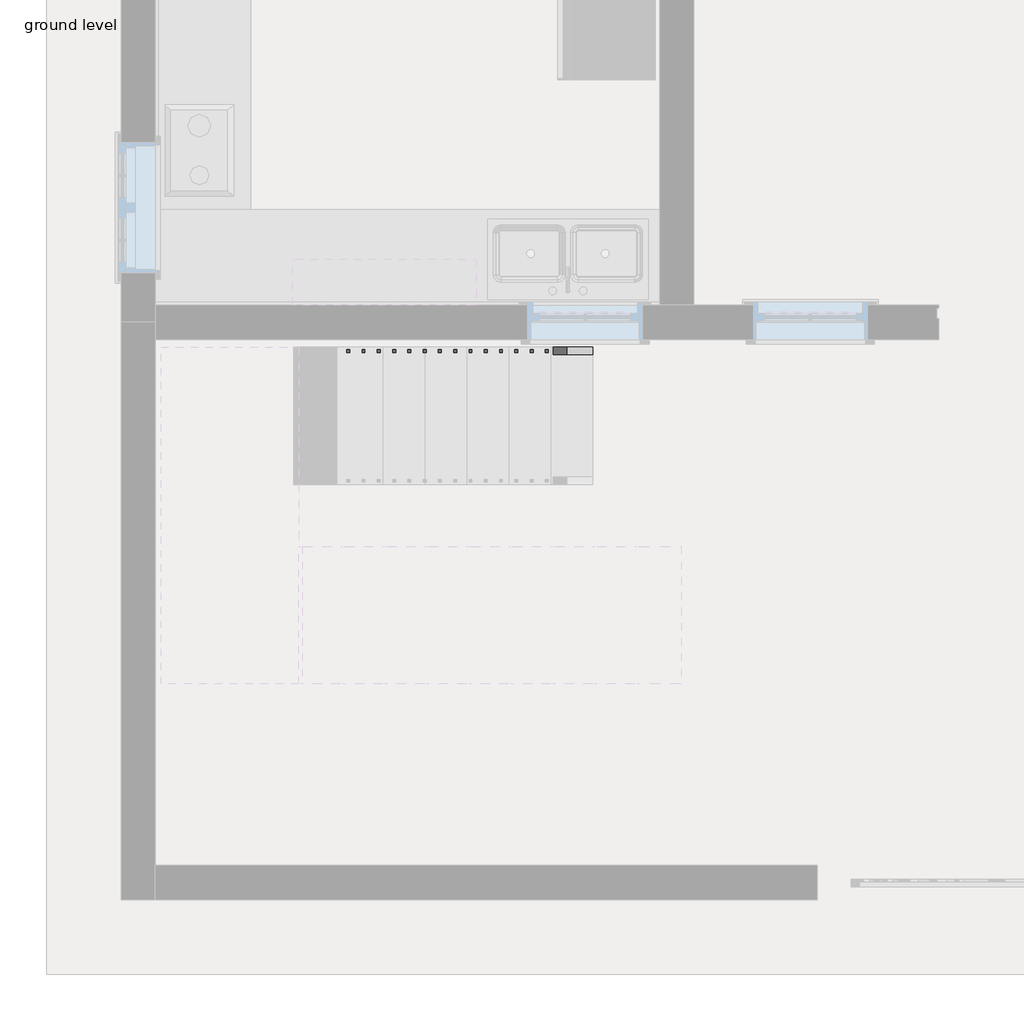
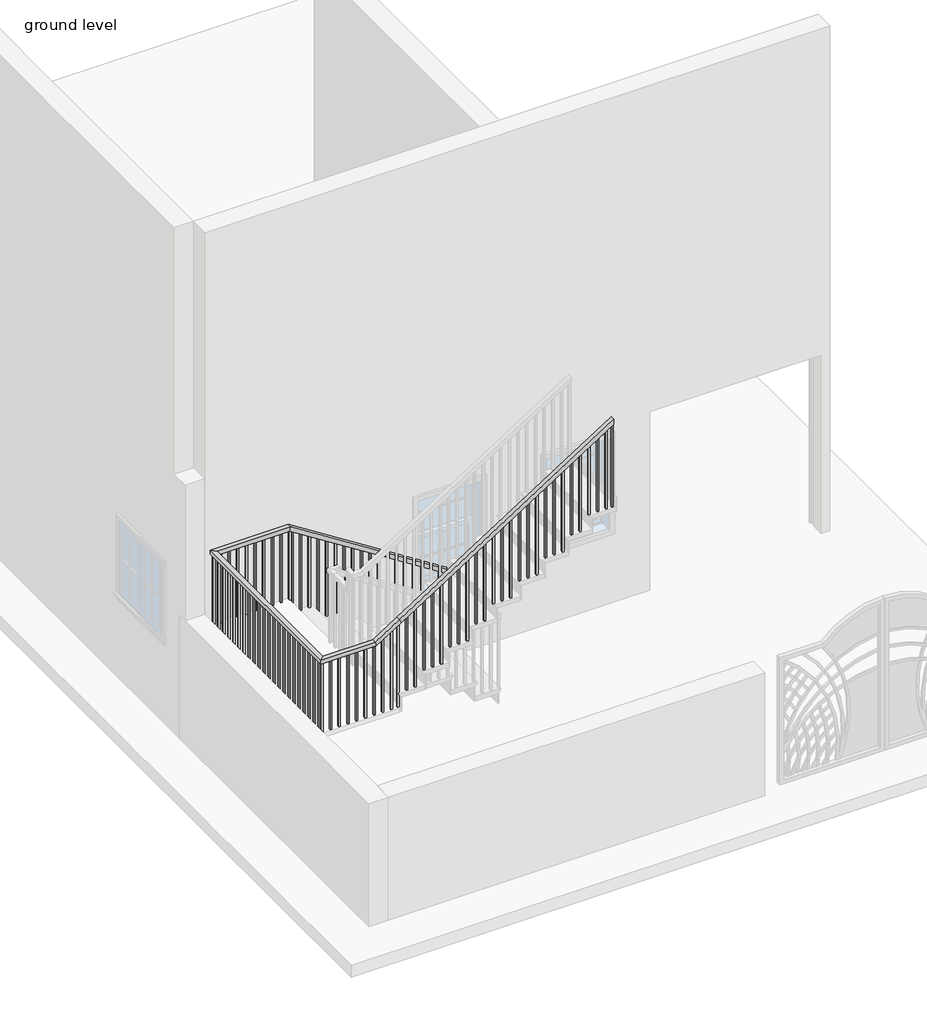
# One storey, part 2 of 3: 1 railing.
"""IFC4 building model written with IfcOpenShell, lengths in millimetres."""

from ifc_helpers import new_model, si_unit, frame, origin, place, context, project, spatial, polyline, outline, extrude, faceted_brep, element, save

model = new_model("IFC4")

# Units and contexts
model_context = context("Model", 3, world=origin())
ifc_project = project(units=[si_unit("LENGTHUNIT", "METRE", prefix="MILLI")], contexts=[model_context])

# Site, building, storey
site = spatial("IfcSite", under=ifc_project)
building = spatial("IfcBuilding", under=site)
storey = spatial("IfcBuildingStorey", under=building, Name="ground level", Elevation=609.6)

# Railing
placement = place(None, origin())
element("IfcRailing", 1, ObjectType="Handrail - Rectangular", at=placement, inside=storey, context=model_context, shape_type="SolidModel", body=[
    faceted_brep([(31519.2316163, 9231.5980552, 1701.8), (31519.2316163, 9231.5980552, 1641.586276), (31519.2316163, 9282.3980552, 1641.586276), (31519.2316163, 9282.3980552, 1701.8), (29563.4316163, 9231.5980552, 2946.4), (29548.6386214, 9231.5980552, 2895.6), (29548.6386214, 9282.3980552, 2895.6), (29563.4316163, 9282.3980552, 2946.4), (28699.8316163, 9231.5980552, 2946.4), (28699.8316163, 9231.5980552, 2895.6), (28649.0316163, 9282.3980552, 2895.6), (28649.0316163, 9282.3980552, 2946.4), (28699.8316163, 7091.6480552, 2946.4), (28699.8316163, 7091.6480552, 2895.6), (28649.0316163, 7040.8480552, 2895.6), (28649.0316163, 7040.8480552, 2946.4), (29284.0316163, 7091.6480552, 2946.4), (29298.8246113, 7091.6480552, 2895.6), (29298.8246113, 7040.8480552, 2895.6), (29284.0316163, 7040.8480552, 2946.4), (29563.4316163, 7091.6480552, 3124.2), (29590.7048913, 7091.6480552, 3081.3419964), (29590.7048913, 7040.8480552, 3081.3419964), (29563.4316163, 7040.8480552, 3124.2), (32078.0316163, 7091.6480552, 4724.4), (32078.0316163, 7040.8480552, 4724.4), (32078.0316163, 7040.8480552, 4664.186276), (32078.0316163, 7091.6480552, 4664.186276)], [[[0, 1, 2, 3]], [[1, 0, 4, 5]], [[2, 1, 5, 6]], [[3, 2, 6, 7]], [[0, 3, 7, 4]], [[5, 4, 8, 9]], [[6, 5, 9, 10]], [[7, 6, 10, 11]], [[4, 7, 11, 8]], [[9, 8, 12, 13]], [[10, 9, 13, 14]], [[11, 10, 14, 15]], [[8, 11, 15, 12]], [[13, 12, 16, 17]], [[14, 13, 17, 18]], [[15, 14, 18, 19]], [[12, 15, 19, 16]], [[17, 16, 20, 21]], [[18, 17, 21, 22]], [[19, 18, 22, 23]], [[16, 19, 23, 20]], [[24, 25, 26, 27]], [[21, 20, 24, 27]], [[22, 21, 27, 26]], [[23, 22, 26, 25]], [[20, 23, 25, 24]]]),
    extrude(outline(polyline([(4621.7567305, 32011.3566163), (4609.6340032, 31992.3066163), (3632.2, 31992.3066163), (3632.2, 32011.3566163), (4621.7567305, 32011.3566163)])), frame((0.0, 7056.7230552, 0.0), z_axis=(0.0, 1.0, 0.0), x_axis=(0.0, 0.0, 1.0)), (0.0, 0.0, 1.0), 19.05),
    extrude(outline(polyline([(4557.1021851, 31909.7566163), (4544.9794578, 31890.7066163), (3632.2, 31890.7066163), (3632.2, 31909.7566163), (4557.1021851, 31909.7566163)])), frame((0.0, 7056.7230552, 0.0), z_axis=(0.0, 1.0, 0.0), x_axis=(0.0, 0.0, 1.0)), (0.0, 0.0, 1.0), 19.05),
    extrude(outline(polyline([(4492.4476396, 31808.1566163), (4480.3249123, 31789.1066163), (3632.2, 31789.1066163), (3632.2, 31808.1566163), (4492.4476396, 31808.1566163)])), frame((0.0, 7056.7230552, 0.0), z_axis=(0.0, 1.0, 0.0), x_axis=(0.0, 0.0, 1.0)), (0.0, 0.0, 1.0), 19.05),
    extrude(outline(polyline([(4427.7930941, 31706.5566163), (4415.6703669, 31687.5066163), (3454.4, 31687.5066163), (3454.4, 31706.5566163), (4427.7930941, 31706.5566163)])), frame((0.0, 7056.7230552, 0.0), z_axis=(0.0, 1.0, 0.0), x_axis=(0.0, 0.0, 1.0)), (0.0, 0.0, 1.0), 19.05),
    extrude(outline(polyline([(4363.1385487, 31604.9566163), (4351.0158214, 31585.9066163), (3454.4, 31585.9066163), (3454.4, 31604.9566163), (4363.1385487, 31604.9566163)])), frame((0.0, 7056.7230552, 0.0), z_axis=(0.0, 1.0, 0.0), x_axis=(0.0, 0.0, 1.0)), (0.0, 0.0, 1.0), 19.05),
    extrude(outline(polyline([(4298.4840032, 31503.3566163), (4286.361276, 31484.3066163), (3276.6, 31484.3066163), (3276.6, 31503.3566163), (4298.4840032, 31503.3566163)])), frame((0.0, 7056.7230552, 0.0), z_axis=(0.0, 1.0, 0.0), x_axis=(0.0, 0.0, 1.0)), (0.0, 0.0, 1.0), 19.05),
    extrude(outline(polyline([(4233.8294578, 31401.7566163), (4221.7067305, 31382.7066163), (3276.6, 31382.7066163), (3276.6, 31401.7566163), (4233.8294578, 31401.7566163)])), frame((0.0, 7056.7230552, 0.0), z_axis=(0.0, 1.0, 0.0), x_axis=(0.0, 0.0, 1.0)), (0.0, 0.0, 1.0), 19.05),
    extrude(outline(polyline([(4169.1749123, 31300.1566163), (4157.0521851, 31281.1066163), (3276.6, 31281.1066163), (3276.6, 31300.1566163), (4169.1749123, 31300.1566163)])), frame((0.0, 7056.7230552, 0.0), z_axis=(0.0, 1.0, 0.0), x_axis=(0.0, 0.0, 1.0)), (0.0, 0.0, 1.0), 19.05),
    extrude(outline(polyline([(4104.5203669, 31198.5566163), (4092.3976396, 31179.5066163), (3098.8, 31179.5066163), (3098.8, 31198.5566163), (4104.5203669, 31198.5566163)])), frame((0.0, 7056.7230552, 0.0), z_axis=(0.0, 1.0, 0.0), x_axis=(0.0, 0.0, 1.0)), (0.0, 0.0, 1.0), 19.05),
    extrude(outline(polyline([(4039.8658214, 31096.9566163), (4027.7430941, 31077.9066163), (3098.8, 31077.9066163), (3098.8, 31096.9566163), (4039.8658214, 31096.9566163)])), frame((0.0, 7056.7230552, 0.0), z_axis=(0.0, 1.0, 0.0), x_axis=(0.0, 0.0, 1.0)), (0.0, 0.0, 1.0), 19.05),
    extrude(outline(polyline([(3975.211276, 30995.3566163), (3963.0885487, 30976.3066163), (3098.8, 30976.3066163), (3098.8, 30995.3566163), (3975.211276, 30995.3566163)])), frame((0.0, 7056.7230552, 0.0), z_axis=(0.0, 1.0, 0.0), x_axis=(0.0, 0.0, 1.0)), (0.0, 0.0, 1.0), 19.05),
    extrude(outline(polyline([(3910.5567305, 30893.7566163), (3898.4340032, 30874.7066163), (2921.0, 30874.7066163), (2921.0, 30893.7566163), (3910.5567305, 30893.7566163)])), frame((0.0, 7056.7230552, 0.0), z_axis=(0.0, 1.0, 0.0), x_axis=(0.0, 0.0, 1.0)), (0.0, 0.0, 1.0), 19.05),
    extrude(outline(polyline([(3845.9021851, 30792.1566163), (3833.7794578, 30773.1066163), (2921.0, 30773.1066163), (2921.0, 30792.1566163), (3845.9021851, 30792.1566163)])), frame((0.0, 7056.7230552, 0.0), z_axis=(0.0, 1.0, 0.0), x_axis=(0.0, 0.0, 1.0)), (0.0, 0.0, 1.0), 19.05),
    extrude(outline(polyline([(3781.2476396, 30690.5566163), (3769.1249123, 30671.5066163), (2921.0, 30671.5066163), (2921.0, 30690.5566163), (3781.2476396, 30690.5566163)])), frame((0.0, 7056.7230552, 0.0), z_axis=(0.0, 1.0, 0.0), x_axis=(0.0, 0.0, 1.0)), (0.0, 0.0, 1.0), 19.05),
    extrude(outline(polyline([(3716.5930941, 30588.9566163), (3704.4703669, 30569.9066163), (2743.2, 30569.9066163), (2743.2, 30588.9566163), (3716.5930941, 30588.9566163)])), frame((0.0, 7056.7230552, 0.0), z_axis=(0.0, 1.0, 0.0), x_axis=(0.0, 0.0, 1.0)), (0.0, 0.0, 1.0), 19.05),
    extrude(outline(polyline([(3651.9385487, 30487.3566163), (3639.8158214, 30468.3066163), (2743.2, 30468.3066163), (2743.2, 30487.3566163), (3651.9385487, 30487.3566163)])), frame((0.0, 7056.7230552, 0.0), z_axis=(0.0, 1.0, 0.0), x_axis=(0.0, 0.0, 1.0)), (0.0, 0.0, 1.0), 19.05),
    extrude(outline(polyline([(3587.2840032, 30385.7566163), (3575.161276, 30366.7066163), (2565.4, 30366.7066163), (2565.4, 30385.7566163), (3587.2840032, 30385.7566163)])), frame((0.0, 7056.7230552, 0.0), z_axis=(0.0, 1.0, 0.0), x_axis=(0.0, 0.0, 1.0)), (0.0, 0.0, 1.0), 19.05),
    extrude(outline(polyline([(3522.6294578, 30284.1566163), (3510.5067305, 30265.1066163), (2565.4, 30265.1066163), (2565.4, 30284.1566163), (3522.6294578, 30284.1566163)])), frame((0.0, 7056.7230552, 0.0), z_axis=(0.0, 1.0, 0.0), x_axis=(0.0, 0.0, 1.0)), (0.0, 0.0, 1.0), 19.05),
    extrude(outline(polyline([(3457.9749123, 30182.5566163), (3445.8521851, 30163.5066163), (2565.4, 30163.5066163), (2565.4, 30182.5566163), (3457.9749123, 30182.5566163)])), frame((0.0, 7056.7230552, 0.0), z_axis=(0.0, 1.0, 0.0), x_axis=(0.0, 0.0, 1.0)), (0.0, 0.0, 1.0), 19.05),
    extrude(outline(polyline([(3393.3203669, 30080.9566163), (3381.1976396, 30061.9066163), (2387.6, 30061.9066163), (2387.6, 30080.9566163), (3393.3203669, 30080.9566163)])), frame((0.0, 7056.7230552, 0.0), z_axis=(0.0, 1.0, 0.0), x_axis=(0.0, 0.0, 1.0)), (0.0, 0.0, 1.0), 19.05),
    extrude(outline(polyline([(3328.6658214, 29979.3566163), (3316.5430941, 29960.3066163), (2387.6, 29960.3066163), (2387.6, 29979.3566163), (3328.6658214, 29979.3566163)])), frame((0.0, 7056.7230552, 0.0), z_axis=(0.0, 1.0, 0.0), x_axis=(0.0, 0.0, 1.0)), (0.0, 0.0, 1.0), 19.05),
    extrude(outline(polyline([(3264.011276, 29877.7566163), (3251.8885487, 29858.7066163), (2387.6, 29858.7066163), (2387.6, 29877.7566163), (3264.011276, 29877.7566163)])), frame((0.0, 7056.7230552, 0.0), z_axis=(0.0, 1.0, 0.0), x_axis=(0.0, 0.0, 1.0)), (0.0, 0.0, 1.0), 19.05),
    extrude(outline(polyline([(3199.3567305, 29776.1566163), (3187.2340032, 29757.1066163), (2209.8, 29757.1066163), (2209.8, 29776.1566163), (3199.3567305, 29776.1566163)])), frame((0.0, 7056.7230552, 0.0), z_axis=(0.0, 1.0, 0.0), x_axis=(0.0, 0.0, 1.0)), (0.0, 0.0, 1.0), 19.05),
    extrude(outline(polyline([(3134.7021851, 29674.5566163), (3122.5794578, 29655.5066163), (2209.8, 29655.5066163), (2209.8, 29674.5566163), (3134.7021851, 29674.5566163)])), frame((0.0, 7056.7230552, 0.0), z_axis=(0.0, 1.0, 0.0), x_axis=(0.0, 0.0, 1.0)), (0.0, 0.0, 1.0), 19.05),
    extrude(outline(polyline([(3021.5567305, 29496.7566163), (3009.4340032, 29477.7066163), (2032.0, 29477.7066163), (2032.0, 29496.7566163), (3021.5567305, 29496.7566163)])), frame((0.0, 7056.7230552, 0.0), z_axis=(0.0, 1.0, 0.0), x_axis=(0.0, 0.0, 1.0)), (0.0, 0.0, 1.0), 19.05),
    extrude(outline(polyline([(2956.9021851, 29395.1566163), (2944.7794578, 29376.1066163), (2032.0, 29376.1066163), (2032.0, 29395.1566163), (2956.9021851, 29395.1566163)])), frame((0.0, 7056.7230552, 0.0), z_axis=(0.0, 1.0, 0.0), x_axis=(0.0, 0.0, 1.0)), (0.0, 0.0, 1.0), 19.05),
    extrude(outline(polyline([(29274.5066163, 7056.7230552), (29274.5066163, 7075.7730552), (29293.5566163, 7075.7730552), (29293.5566163, 7056.7230552), (29274.5066163, 7056.7230552)])), frame((0.0, 0.0, 2032.0), z_axis=(0.0, 0.0, 1.0), x_axis=(1.0, 0.0, 0.0)), (0.0, 0.0, 1.0), 863.6),
    extrude(outline(polyline([(29172.9066163, 7056.7230552), (29172.9066163, 7075.7730552), (29191.9566163, 7075.7730552), (29191.9566163, 7056.7230552), (29172.9066163, 7056.7230552)])), frame((0.0, 0.0, 2032.0), z_axis=(0.0, 0.0, 1.0), x_axis=(1.0, 0.0, 0.0)), (0.0, 0.0, 1.0), 863.6),
    extrude(outline(polyline([(29071.3066163, 7056.7230552), (29071.3066163, 7075.7730552), (29090.3566163, 7075.7730552), (29090.3566163, 7056.7230552), (29071.3066163, 7056.7230552)])), frame((0.0, 0.0, 2032.0), z_axis=(0.0, 0.0, 1.0), x_axis=(1.0, 0.0, 0.0)), (0.0, 0.0, 1.0), 863.6),
    extrude(outline(polyline([(28969.7066163, 7056.7230552), (28969.7066163, 7075.7730552), (28988.7566163, 7075.7730552), (28988.7566163, 7056.7230552), (28969.7066163, 7056.7230552)])), frame((0.0, 0.0, 2032.0), z_axis=(0.0, 0.0, 1.0), x_axis=(1.0, 0.0, 0.0)), (0.0, 0.0, 1.0), 863.6),
    extrude(outline(polyline([(28868.1066163, 7056.7230552), (28868.1066163, 7075.7730552), (28887.1566163, 7075.7730552), (28887.1566163, 7056.7230552), (28868.1066163, 7056.7230552)])), frame((0.0, 0.0, 2032.0), z_axis=(0.0, 0.0, 1.0), x_axis=(1.0, 0.0, 0.0)), (0.0, 0.0, 1.0), 863.6),
    extrude(outline(polyline([(28766.5066163, 7056.7230552), (28766.5066163, 7075.7730552), (28785.5566163, 7075.7730552), (28785.5566163, 7056.7230552), (28766.5066163, 7056.7230552)])), frame((0.0, 0.0, 2032.0), z_axis=(0.0, 0.0, 1.0), x_axis=(1.0, 0.0, 0.0)), (0.0, 0.0, 1.0), 863.6),
    extrude(outline(polyline([(28664.9066163, 7132.9230552), (28683.9566163, 7132.9230552), (28683.9566163, 7113.8730552), (28664.9066163, 7113.8730552), (28664.9066163, 7132.9230552)])), frame((0.0, 0.0, 2032.0), z_axis=(0.0, 0.0, 1.0), x_axis=(1.0, 0.0, 0.0)), (0.0, 0.0, 1.0), 863.6),
    extrude(outline(polyline([(28664.9066163, 7234.5230552), (28683.9566163, 7234.5230552), (28683.9566163, 7215.4730552), (28664.9066163, 7215.4730552), (28664.9066163, 7234.5230552)])), frame((0.0, 0.0, 2032.0), z_axis=(0.0, 0.0, 1.0), x_axis=(1.0, 0.0, 0.0)), (0.0, 0.0, 1.0), 863.6),
    extrude(outline(polyline([(28664.9066163, 7336.1230552), (28683.9566163, 7336.1230552), (28683.9566163, 7317.0730552), (28664.9066163, 7317.0730552), (28664.9066163, 7336.1230552)])), frame((0.0, 0.0, 2032.0), z_axis=(0.0, 0.0, 1.0), x_axis=(1.0, 0.0, 0.0)), (0.0, 0.0, 1.0), 863.6),
    extrude(outline(polyline([(28664.9066163, 7437.7230552), (28683.9566163, 7437.7230552), (28683.9566163, 7418.6730552), (28664.9066163, 7418.6730552), (28664.9066163, 7437.7230552)])), frame((0.0, 0.0, 2032.0), z_axis=(0.0, 0.0, 1.0), x_axis=(1.0, 0.0, 0.0)), (0.0, 0.0, 1.0), 863.6),
    extrude(outline(polyline([(28664.9066163, 7539.3230552), (28683.9566163, 7539.3230552), (28683.9566163, 7520.2730552), (28664.9066163, 7520.2730552), (28664.9066163, 7539.3230552)])), frame((0.0, 0.0, 2032.0), z_axis=(0.0, 0.0, 1.0), x_axis=(1.0, 0.0, 0.0)), (0.0, 0.0, 1.0), 863.6),
    extrude(outline(polyline([(28664.9066163, 7640.9230552), (28683.9566163, 7640.9230552), (28683.9566163, 7621.8730552), (28664.9066163, 7621.8730552), (28664.9066163, 7640.9230552)])), frame((0.0, 0.0, 2032.0), z_axis=(0.0, 0.0, 1.0), x_axis=(1.0, 0.0, 0.0)), (0.0, 0.0, 1.0), 863.6),
    extrude(outline(polyline([(28664.9066163, 7742.5230552), (28683.9566163, 7742.5230552), (28683.9566163, 7723.4730552), (28664.9066163, 7723.4730552), (28664.9066163, 7742.5230552)])), frame((0.0, 0.0, 2032.0), z_axis=(0.0, 0.0, 1.0), x_axis=(1.0, 0.0, 0.0)), (0.0, 0.0, 1.0), 863.6),
    extrude(outline(polyline([(28664.9066163, 7844.1230552), (28683.9566163, 7844.1230552), (28683.9566163, 7825.0730552), (28664.9066163, 7825.0730552), (28664.9066163, 7844.1230552)])), frame((0.0, 0.0, 2032.0), z_axis=(0.0, 0.0, 1.0), x_axis=(1.0, 0.0, 0.0)), (0.0, 0.0, 1.0), 863.6),
    extrude(outline(polyline([(28664.9066163, 7945.7230552), (28683.9566163, 7945.7230552), (28683.9566163, 7926.6730552), (28664.9066163, 7926.6730552), (28664.9066163, 7945.7230552)])), frame((0.0, 0.0, 2032.0), z_axis=(0.0, 0.0, 1.0), x_axis=(1.0, 0.0, 0.0)), (0.0, 0.0, 1.0), 863.6),
    extrude(outline(polyline([(28664.9066163, 8047.3230552), (28683.9566163, 8047.3230552), (28683.9566163, 8028.2730552), (28664.9066163, 8028.2730552), (28664.9066163, 8047.3230552)])), frame((0.0, 0.0, 2032.0), z_axis=(0.0, 0.0, 1.0), x_axis=(1.0, 0.0, 0.0)), (0.0, 0.0, 1.0), 863.6),
    extrude(outline(polyline([(28664.9066163, 8148.9230552), (28683.9566163, 8148.9230552), (28683.9566163, 8129.8730552), (28664.9066163, 8129.8730552), (28664.9066163, 8148.9230552)])), frame((0.0, 0.0, 2032.0), z_axis=(0.0, 0.0, 1.0), x_axis=(1.0, 0.0, 0.0)), (0.0, 0.0, 1.0), 863.6),
    extrude(outline(polyline([(28664.9066163, 8250.5230552), (28683.9566163, 8250.5230552), (28683.9566163, 8231.4730552), (28664.9066163, 8231.4730552), (28664.9066163, 8250.5230552)])), frame((0.0, 0.0, 2032.0), z_axis=(0.0, 0.0, 1.0), x_axis=(1.0, 0.0, 0.0)), (0.0, 0.0, 1.0), 863.6),
    extrude(outline(polyline([(28664.9066163, 8352.1230552), (28683.9566163, 8352.1230552), (28683.9566163, 8333.0730552), (28664.9066163, 8333.0730552), (28664.9066163, 8352.1230552)])), frame((0.0, 0.0, 2032.0), z_axis=(0.0, 0.0, 1.0), x_axis=(1.0, 0.0, 0.0)), (0.0, 0.0, 1.0), 863.6),
    extrude(outline(polyline([(28664.9066163, 8453.7230552), (28683.9566163, 8453.7230552), (28683.9566163, 8434.6730552), (28664.9066163, 8434.6730552), (28664.9066163, 8453.7230552)])), frame((0.0, 0.0, 2032.0), z_axis=(0.0, 0.0, 1.0), x_axis=(1.0, 0.0, 0.0)), (0.0, 0.0, 1.0), 863.6),
    extrude(outline(polyline([(28664.9066163, 8555.3230552), (28683.9566163, 8555.3230552), (28683.9566163, 8536.2730552), (28664.9066163, 8536.2730552), (28664.9066163, 8555.3230552)])), frame((0.0, 0.0, 2032.0), z_axis=(0.0, 0.0, 1.0), x_axis=(1.0, 0.0, 0.0)), (0.0, 0.0, 1.0), 863.6),
    extrude(outline(polyline([(28664.9066163, 8656.9230552), (28683.9566163, 8656.9230552), (28683.9566163, 8637.8730552), (28664.9066163, 8637.8730552), (28664.9066163, 8656.9230552)])), frame((0.0, 0.0, 2032.0), z_axis=(0.0, 0.0, 1.0), x_axis=(1.0, 0.0, 0.0)), (0.0, 0.0, 1.0), 863.6),
    extrude(outline(polyline([(28664.9066163, 8758.5230552), (28683.9566163, 8758.5230552), (28683.9566163, 8739.4730552), (28664.9066163, 8739.4730552), (28664.9066163, 8758.5230552)])), frame((0.0, 0.0, 2032.0), z_axis=(0.0, 0.0, 1.0), x_axis=(1.0, 0.0, 0.0)), (0.0, 0.0, 1.0), 863.6),
    extrude(outline(polyline([(28664.9066163, 8860.1230552), (28683.9566163, 8860.1230552), (28683.9566163, 8841.0730552), (28664.9066163, 8841.0730552), (28664.9066163, 8860.1230552)])), frame((0.0, 0.0, 2032.0), z_axis=(0.0, 0.0, 1.0), x_axis=(1.0, 0.0, 0.0)), (0.0, 0.0, 1.0), 863.6),
    extrude(outline(polyline([(28664.9066163, 8961.7230552), (28683.9566163, 8961.7230552), (28683.9566163, 8942.6730552), (28664.9066163, 8942.6730552), (28664.9066163, 8961.7230552)])), frame((0.0, 0.0, 2032.0), z_axis=(0.0, 0.0, 1.0), x_axis=(1.0, 0.0, 0.0)), (0.0, 0.0, 1.0), 863.6),
    extrude(outline(polyline([(28664.9066163, 9063.3230552), (28683.9566163, 9063.3230552), (28683.9566163, 9044.2730552), (28664.9066163, 9044.2730552), (28664.9066163, 9063.3230552)])), frame((0.0, 0.0, 2032.0), z_axis=(0.0, 0.0, 1.0), x_axis=(1.0, 0.0, 0.0)), (0.0, 0.0, 1.0), 863.6),
    extrude(outline(polyline([(28664.9066163, 9164.9230552), (28683.9566163, 9164.9230552), (28683.9566163, 9145.8730552), (28664.9066163, 9145.8730552), (28664.9066163, 9164.9230552)])), frame((0.0, 0.0, 2032.0), z_axis=(0.0, 0.0, 1.0), x_axis=(1.0, 0.0, 0.0)), (0.0, 0.0, 1.0), 863.6),
    extrude(outline(polyline([(28760.1566163, 9266.5230552), (28760.1566163, 9247.4730552), (28741.1066163, 9247.4730552), (28741.1066163, 9266.5230552), (28760.1566163, 9266.5230552)])), frame((0.0, 0.0, 2032.0), z_axis=(0.0, 0.0, 1.0), x_axis=(1.0, 0.0, 0.0)), (0.0, 0.0, 1.0), 863.6),
    extrude(outline(polyline([(28861.7566163, 9266.5230552), (28861.7566163, 9247.4730552), (28842.7066163, 9247.4730552), (28842.7066163, 9266.5230552), (28861.7566163, 9266.5230552)])), frame((0.0, 0.0, 2032.0), z_axis=(0.0, 0.0, 1.0), x_axis=(1.0, 0.0, 0.0)), (0.0, 0.0, 1.0), 863.6),
    extrude(outline(polyline([(28963.3566163, 9266.5230552), (28963.3566163, 9247.4730552), (28944.3066163, 9247.4730552), (28944.3066163, 9266.5230552), (28963.3566163, 9266.5230552)])), frame((0.0, 0.0, 2032.0), z_axis=(0.0, 0.0, 1.0), x_axis=(1.0, 0.0, 0.0)), (0.0, 0.0, 1.0), 863.6),
    extrude(outline(polyline([(29064.9566163, 9266.5230552), (29064.9566163, 9247.4730552), (29045.9066163, 9247.4730552), (29045.9066163, 9266.5230552), (29064.9566163, 9266.5230552)])), frame((0.0, 0.0, 2032.0), z_axis=(0.0, 0.0, 1.0), x_axis=(1.0, 0.0, 0.0)), (0.0, 0.0, 1.0), 863.6),
    extrude(outline(polyline([(29166.5566163, 9266.5230552), (29166.5566163, 9247.4730552), (29147.5066163, 9247.4730552), (29147.5066163, 9266.5230552), (29166.5566163, 9266.5230552)])), frame((0.0, 0.0, 2032.0), z_axis=(0.0, 0.0, 1.0), x_axis=(1.0, 0.0, 0.0)), (0.0, 0.0, 1.0), 863.6),
    extrude(outline(polyline([(29268.1566163, 9266.5230552), (29268.1566163, 9247.4730552), (29249.1066163, 9247.4730552), (29249.1066163, 9266.5230552), (29268.1566163, 9266.5230552)])), frame((0.0, 0.0, 2032.0), z_axis=(0.0, 0.0, 1.0), x_axis=(1.0, 0.0, 0.0)), (0.0, 0.0, 1.0), 863.6),
    extrude(outline(polyline([(29369.7566163, 9266.5230552), (29369.7566163, 9247.4730552), (29350.7066163, 9247.4730552), (29350.7066163, 9266.5230552), (29369.7566163, 9266.5230552)])), frame((0.0, 0.0, 2032.0), z_axis=(0.0, 0.0, 1.0), x_axis=(1.0, 0.0, 0.0)), (0.0, 0.0, 1.0), 863.6),
    extrude(outline(polyline([(29471.3566163, 9266.5230552), (29471.3566163, 9247.4730552), (29452.3066163, 9247.4730552), (29452.3066163, 9266.5230552), (29471.3566163, 9266.5230552)])), frame((0.0, 0.0, 2032.0), z_axis=(0.0, 0.0, 1.0), x_axis=(1.0, 0.0, 0.0)), (0.0, 0.0, 1.0), 863.6),
    extrude(outline(polyline([(2863.961276, 29598.3566163), (2876.0840032, 29579.3066163), (1854.2, 29579.3066163), (1854.2, 29598.3566163), (2863.961276, 29598.3566163)])), frame((0.0, 9247.4730552, 0.0), z_axis=(0.0, 1.0, 0.0), x_axis=(0.0, 0.0, 1.0)), (0.0, 0.0, 1.0), 19.05),
    extrude(outline(polyline([(2799.3067305, 29699.9566163), (2811.4294578, 29680.9066163), (1854.2, 29680.9066163), (1854.2, 29699.9566163), (2799.3067305, 29699.9566163)])), frame((0.0, 9247.4730552, 0.0), z_axis=(0.0, 1.0, 0.0), x_axis=(0.0, 0.0, 1.0)), (0.0, 0.0, 1.0), 19.05),
    extrude(outline(polyline([(2734.6521851, 29801.5566163), (2746.7749123, 29782.5066163), (1854.2, 29782.5066163), (1854.2, 29801.5566163), (2734.6521851, 29801.5566163)])), frame((0.0, 9247.4730552, 0.0), z_axis=(0.0, 1.0, 0.0), x_axis=(0.0, 0.0, 1.0)), (0.0, 0.0, 1.0), 19.05),
    extrude(outline(polyline([(2669.9976396, 29903.1566163), (2682.1203669, 29884.1066163), (1676.4, 29884.1066163), (1676.4, 29903.1566163), (2669.9976396, 29903.1566163)])), frame((0.0, 9247.4730552, 0.0), z_axis=(0.0, 1.0, 0.0), x_axis=(0.0, 0.0, 1.0)), (0.0, 0.0, 1.0), 19.05),
    extrude(outline(polyline([(2605.3430941, 30004.7566163), (2617.4658214, 29985.7066163), (1676.4, 29985.7066163), (1676.4, 30004.7566163), (2605.3430941, 30004.7566163)])), frame((0.0, 9247.4730552, 0.0), z_axis=(0.0, 1.0, 0.0), x_axis=(0.0, 0.0, 1.0)), (0.0, 0.0, 1.0), 19.05),
    extrude(outline(polyline([(2540.6885487, 30106.3566163), (2552.811276, 30087.3066163), (1676.4, 30087.3066163), (1676.4, 30106.3566163), (2540.6885487, 30106.3566163)])), frame((0.0, 9247.4730552, 0.0), z_axis=(0.0, 1.0, 0.0), x_axis=(0.0, 0.0, 1.0)), (0.0, 0.0, 1.0), 19.05),
    extrude(outline(polyline([(2476.0340032, 30207.9566163), (2488.1567305, 30188.9066163), (1498.6, 30188.9066163), (1498.6, 30207.9566163), (2476.0340032, 30207.9566163)])), frame((0.0, 9247.4730552, 0.0), z_axis=(0.0, 1.0, 0.0), x_axis=(0.0, 0.0, 1.0)), (0.0, 0.0, 1.0), 19.05),
    extrude(outline(polyline([(2411.3794578, 30309.5566163), (2423.5021851, 30290.5066163), (1498.6, 30290.5066163), (1498.6, 30309.5566163), (2411.3794578, 30309.5566163)])), frame((0.0, 9247.4730552, 0.0), z_axis=(0.0, 1.0, 0.0), x_axis=(0.0, 0.0, 1.0)), (0.0, 0.0, 1.0), 19.05),
    extrude(outline(polyline([(2346.7249123, 30411.1566163), (2358.8476396, 30392.1066163), (1498.6, 30392.1066163), (1498.6, 30411.1566163), (2346.7249123, 30411.1566163)])), frame((0.0, 9247.4730552, 0.0), z_axis=(0.0, 1.0, 0.0), x_axis=(0.0, 0.0, 1.0)), (0.0, 0.0, 1.0), 19.05),
    extrude(outline(polyline([(2282.0703669, 30512.7566163), (2294.1930941, 30493.7066163), (1320.8, 30493.7066163), (1320.8, 30512.7566163), (2282.0703669, 30512.7566163)])), frame((0.0, 9247.4730552, 0.0), z_axis=(0.0, 1.0, 0.0), x_axis=(0.0, 0.0, 1.0)), (0.0, 0.0, 1.0), 19.05),
    extrude(outline(polyline([(2217.4158214, 30614.3566163), (2229.5385487, 30595.3066163), (1320.8, 30595.3066163), (1320.8, 30614.3566163), (2217.4158214, 30614.3566163)])), frame((0.0, 9247.4730552, 0.0), z_axis=(0.0, 1.0, 0.0), x_axis=(0.0, 0.0, 1.0)), (0.0, 0.0, 1.0), 19.05),
    extrude(outline(polyline([(2152.761276, 30715.9566163), (2164.8840032, 30696.9066163), (1143.0, 30696.9066163), (1143.0, 30715.9566163), (2152.761276, 30715.9566163)])), frame((0.0, 9247.4730552, 0.0), z_axis=(0.0, 1.0, 0.0), x_axis=(0.0, 0.0, 1.0)), (0.0, 0.0, 1.0), 19.05),
    extrude(outline(polyline([(2088.1067305, 30817.5566163), (2100.2294578, 30798.5066163), (1143.0, 30798.5066163), (1143.0, 30817.5566163), (2088.1067305, 30817.5566163)])), frame((0.0, 9247.4730552, 0.0), z_axis=(0.0, 1.0, 0.0), x_axis=(0.0, 0.0, 1.0)), (0.0, 0.0, 1.0), 19.05),
    extrude(outline(polyline([(2023.4521851, 30919.1566163), (2035.5749123, 30900.1066163), (1143.0, 30900.1066163), (1143.0, 30919.1566163), (2023.4521851, 30919.1566163)])), frame((0.0, 9247.4730552, 0.0), z_axis=(0.0, 1.0, 0.0), x_axis=(0.0, 0.0, 1.0)), (0.0, 0.0, 1.0), 19.05),
    extrude(outline(polyline([(1958.7976396, 31020.7566163), (1970.9203669, 31001.7066163), (965.2, 31001.7066163), (965.2, 31020.7566163), (1958.7976396, 31020.7566163)])), frame((0.0, 9247.4730552, 0.0), z_axis=(0.0, 1.0, 0.0), x_axis=(0.0, 0.0, 1.0)), (0.0, 0.0, 1.0), 19.05),
    extrude(outline(polyline([(1894.1430941, 31122.3566163), (1906.2658214, 31103.3066163), (965.2, 31103.3066163), (965.2, 31122.3566163), (1894.1430941, 31122.3566163)])), frame((0.0, 9247.4730552, 0.0), z_axis=(0.0, 1.0, 0.0), x_axis=(0.0, 0.0, 1.0)), (0.0, 0.0, 1.0), 19.05),
    extrude(outline(polyline([(1829.4885487, 31223.9566163), (1841.611276, 31204.9066163), (965.2, 31204.9066163), (965.2, 31223.9566163), (1829.4885487, 31223.9566163)])), frame((0.0, 9247.4730552, 0.0), z_axis=(0.0, 1.0, 0.0), x_axis=(0.0, 0.0, 1.0)), (0.0, 0.0, 1.0), 19.05),
    extrude(outline(polyline([(1764.8340032, 31325.5566163), (1776.9567305, 31306.5066163), (787.4, 31306.5066163), (787.4, 31325.5566163), (1764.8340032, 31325.5566163)])), frame((0.0, 9247.4730552, 0.0), z_axis=(0.0, 1.0, 0.0), x_axis=(0.0, 0.0, 1.0)), (0.0, 0.0, 1.0), 19.05),
    extrude(outline(polyline([(1700.1794578, 31427.1566163), (1712.3021851, 31408.1066163), (787.4, 31408.1066163), (787.4, 31427.1566163), (1700.1794578, 31427.1566163)])), frame((0.0, 9247.4730552, 0.0), z_axis=(0.0, 1.0, 0.0), x_axis=(0.0, 0.0, 1.0)), (0.0, 0.0, 1.0), 19.05),
    extrude(outline(polyline([(3070.0476396, 29572.9566163), (3057.9249123, 29553.9066163), (2032.0, 29553.9066163), (2032.0, 29572.9566163), (3070.0476396, 29572.9566163)])), frame((0.0, 7056.7230552, 0.0), z_axis=(0.0, 1.0, 0.0), x_axis=(0.0, 0.0, 1.0)), (0.0, 0.0, 1.0), 19.05),
    extrude(outline(polyline([(28664.9066163, 7075.7730552), (28683.9566163, 7075.7730552), (28683.9566163, 7056.7230552), (28664.9066163, 7056.7230552), (28664.9066163, 7075.7730552)])), frame((0.0, 0.0, 2032.0), z_axis=(0.0, 0.0, 1.0), x_axis=(1.0, 0.0, 0.0)), (0.0, 0.0, 1.0), 863.6),
    extrude(outline(polyline([(28683.9566163, 9266.5230552), (28683.9566163, 9247.4730552), (28664.9066163, 9247.4730552), (28664.9066163, 9266.5230552), (28683.9566163, 9266.5230552)])), frame((0.0, 0.0, 2032.0), z_axis=(0.0, 0.0, 1.0), x_axis=(1.0, 0.0, 0.0)), (0.0, 0.0, 1.0), 863.6),
    extrude(outline(polyline([(2880.1249123, 29572.9566163), (2892.2476396, 29553.9066163), (2032.0, 29553.9066163), (2032.0, 29572.9566163), (2880.1249123, 29572.9566163)])), frame((0.0, 9247.4730552, 0.0), z_axis=(0.0, 1.0, 0.0), x_axis=(0.0, 0.0, 1.0)), (0.0, 0.0, 1.0), 19.05),
    extrude(outline(polyline([(4664.186276, 32078.0316163), (4652.0635487, 32058.9816163), (3632.2, 32058.9816163), (3632.2, 32078.0316163), (4664.186276, 32078.0316163)])), frame((0.0, 7056.7230552, 0.0), z_axis=(0.0, 1.0, 0.0), x_axis=(0.0, 0.0, 1.0)), (0.0, 0.0, 1.0), 19.05),
    extrude(outline(polyline([(1641.586276, 31519.2316163), (1653.7090032, 31500.1816163), (787.4, 31500.1816163), (787.4, 31519.2316163), (1641.586276, 31519.2316163)])), frame((0.0, 9247.4730552, 0.0), z_axis=(0.0, 1.0, 0.0), x_axis=(0.0, 0.0, 1.0)), (0.0, 0.0, 1.0), 19.05),
])

save(model, "model.ifc")

# Revit data of these elements
# Type "Handrail - Rectangular"
#   Assembly Code = "C2010400"
#   built-in parameter 1008612 = 0.0416667 (stored number, unit not read)
#   built-in parameter 1008611 = 0.0416667 (stored number, unit not read)
#   built-in parameter 1008609 = 0.333333 (stored number, unit not read)
#   built-in parameter 1008604 = 0.166667 (stored number, unit not read)
#   built-in parameter 1008603 = 0.166667 (stored number, unit not read)
#   Railing Height = 3' - 0"
#   built-in parameter 1008630 = 2
#   built-in parameter 1008610 = 2
#   built-in parameter 1008618 = Baluster - Square : 3/4"
# Element 1 (IfcRailing, "Handrail - Rectangular")
#   Phase Created = New Construction
